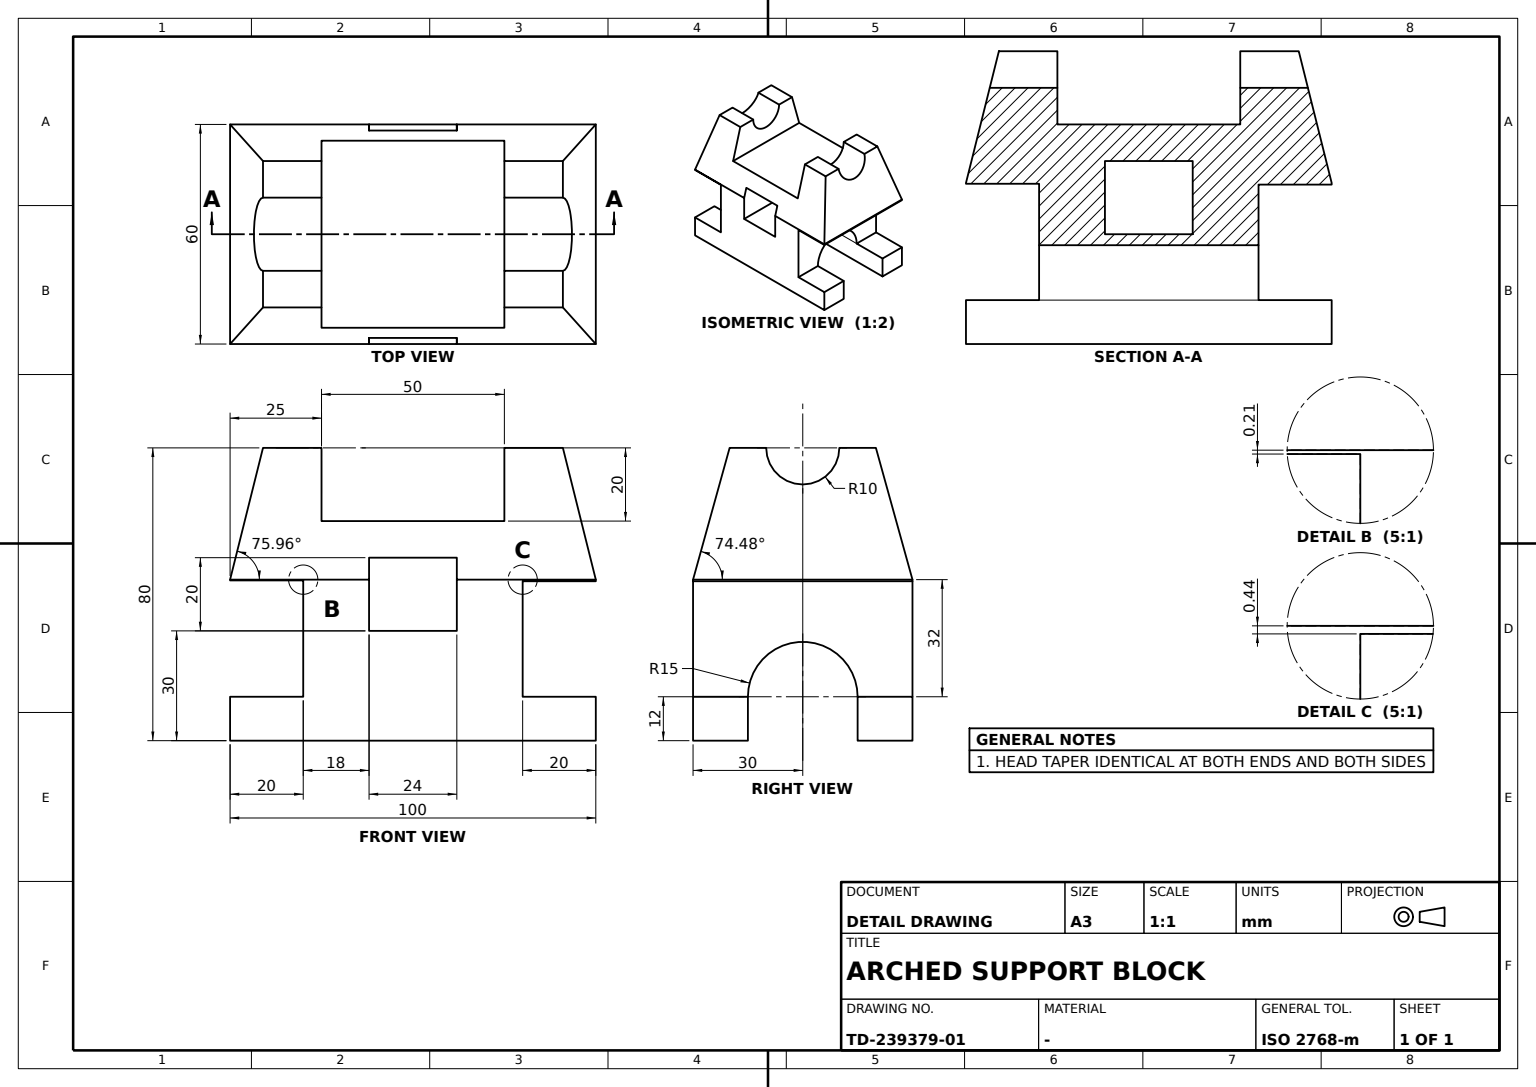
CATIA V5 part; units mm, degrees
sketch "Sketch1" plane through (0, 0, 0) normal (0, 0, 1) x (0, 1, 0)
  line L0 (0, 0) -> (100, 0)
  line L1 (100, 0) -> (100, -60)
  line L2 (100, -60) -> (0, -60)
  line L3 (0, -60) -> (0, 0)
  dimension "length L1" = 60
  dimension "length L2" = 100
  constraint horizontal L0 x-axis
  constraint horizontal L2 x-axis
  constraint vertical L1 y-axis
  constraint vertical L3 y-axis
extrude "Pad1" add sketch "Sketch1" along normal blind 12
sketch "Sketch2" plane through (0, 100, 0) normal (0, 1, 0) x (-1, 0, 0)
  line L0 (-45, 12) -> (-15, 12)
  line L1 (-15, 12) -> (-15, 0)
  line L2 (-15, 0) -> (-45, 0)
  line L3 (-45, 0) -> (-45, 12)
  line L4 (-60, 12) -> (0, 12) construction
  line L5 (-60, 0) -> (0, 0) construction
  dimension "length L0" = 30
  dimension "D2" = 15
  constraint horizontal L0 x-axis
  constraint horizontal L2 x-axis
  constraint vertical L1 y-axis
  constraint vertical L3 y-axis
  constraint coincidence L0 L4
  constraint coincidence L2 L5
extrude "Pocket1" cut sketch "Sketch2" against normal up to next
sketch "Sketch3" plane through (0, 100, 0) normal (0, 1, 0) x (-1, 0, 0)
  arc A0 (-15, 12) -> (-45, 12) centre (-30, 12) ccw
  point P0 (-30, 12)
  line L0 (-15, 12) -> (0, 12)
  point P1 (0, 12)
  line L1 (0, 12) -> (0, 44)
  line L2 (-60, 44) -> (-60, 12)
  point P2 (-60, 12)
  line L3 (-60, 12) -> (-45, 12)
  line L4 (-60, 44) -> (-50, 80)
  line L5 (-50, 80) -> (-10, 80)
  line L6 (-60, 12) -> (0, 12) construction
  line L7 (0, 44) -> (-10, 80)
  dimension "radius A0" = 15
  dimension "D2" = 30
  dimension "length L3" = 15
  dimension "length L0" = 15
  dimension "length L1" = 32
  dimension "length L5" = 40
  constraint coincidence P1 y-axis
  constraint coincidence P2 L0
  constraint coincidence L6 L3
  constraint horizontal L0 x-axis
  constraint horizontal L3 x-axis
  constraint horizontal L5 x-axis
  constraint vertical L1 y-axis
  constraint vertical L2 y-axis
extrude "Pad2" add sketch "Sketch3" against normal blind 100
sketch "Sketch4" plane through (0, 100, 0) normal (0, 1, 0) x (-1, 0, 0)
  arc A0 (-15, 12) -> (-45, 12) centre (-30, 12) ccw
  line L0 (-60, 12) -> (-45, 12)
  line L1 (0, 12) -> (0, 43.56)
  line L2 (0, 43.56) -> (-60, 43.56)
  line L3 (-60, 43.56) -> (-60, 12)
  line L4 (-15, 12) -> (0, 12)
  dimension "radius A0" = 15
  constraint horizontal L0 x-axis
  constraint horizontal L2 x-axis
  constraint horizontal L4 x-axis
  constraint vertical L1 y-axis
  constraint vertical L3 y-axis
  constraint coincidence L0 L4
extrude "Pocket2" cut sketch "Sketch4" against normal blind 20
sketch "Sketch5" plane through (0, 0, 0) normal (0, -1, 0) x (1, 0, 0)
  point P0 (-7.395, 11.9415)
  point P1 (-7.395, -0.0585)
  arc A0 (45, 12) -> (15, 12) centre (30, 12) ccw
  line L0 (0, 12) -> (15, 12)
  line L1 (60, 12) -> (60, 43.7881)
  line L2 (60, 43.7881) -> (0, 43.7881)
  line L3 (0, 43.7881) -> (0, 12)
  line L4 (45, 12) -> (60, 12)
  dimension "radius A0" = 15
  constraint horizontal L0 x-axis
  constraint horizontal L2 x-axis
  constraint horizontal L4 x-axis
  constraint vertical L1 y-axis
  constraint vertical L3 y-axis
  constraint coincidence L0 L4
extrude "Pocket3" cut sketch "Sketch5" against normal blind 20
sketch "Sketch6" plane through (0, 100, 0) normal (0, 1, 0) x (-1, 0, 0)
  arc A0 (-40, 80) -> (-20, 80) centre (-30, 80) ccw
  point P0 (-40, 80)
  point P1 (-20, 80)
  point P2 (-10, 80)
  point P3 (-50, 80)
  dimension "radius A0" = 10
  dimension "distance P1 P2" = 10
  dimension "distance P0 P3" = 10
extrude "Pocket4" cut sketch "Sketch6" against normal up to next material side at (30, 100, 70.05)
sketch "Sketch7" plane through (0, 0, 0) normal (-1, 0, 0) x (0, -1, 0)
  line L0 (-75, 80) -> (-25, 80)
  line L1 (-25, 80) -> (-25, 60)
  line L2 (-25, 60) -> (-75, 60)
  line L3 (-75, 60) -> (-75, 80)
  line L4 (-100, 80) -> (0, 80) construction
  line L5 (0, 44) -> (0, 80) construction
  dimension "length L0" = 50
  dimension "length L1" = 20
  dimension "distance L1 L5" = 25
  constraint horizontal L0 x-axis
  constraint horizontal L2 x-axis
  constraint vertical L1 y-axis
  constraint vertical L3 y-axis
  constraint coincidence L0 L4
extrude "Pocket5" cut sketch "Sketch7" against normal up to next
sketch "Sketch8" plane through (0, 0, 0) normal (-1, 0, 0) x (0, -1, 0)
  line L0 (-100, 80) -> (-91, 80)
  line L1 (-91, 80) -> (-100, 44)
  line L2 (-100, 44) -> (-100, 80)
  line L3 (0, 80) -> (-9, 80)
  line L4 (-9, 80) -> (0, 44)
  line L5 (0, 44) -> (0, 80)
  dimension "length L0" = 9
  constraint horizontal L0 x-axis
  constraint vertical L2 y-axis
extrude "Pocket6" cut sketch "Sketch8" against normal up to next
sketch "Sketch9" plane through (0, 0, 0) normal (-1, 0, 0) x (0, -1, 0)
  line L0 (-62, 50) -> (-38, 50)
  line L1 (-38, 50) -> (-38, 30)
  line L2 (-38, 30) -> (-62, 30)
  line L3 (-62, 30) -> (-62, 50)
  line L4 (-100, 0) -> (0, 0) construction
  dimension "length L0" = 24
  dimension "length L1" = 20
  dimension "distance L2 L4" = 30
  constraint horizontal L0 x-axis
  constraint horizontal L2 x-axis
  constraint vertical L1 y-axis
  constraint vertical L3 y-axis
extrude "Pocket7" cut sketch "Sketch9" against normal up to next
properties part number "catia 22"
